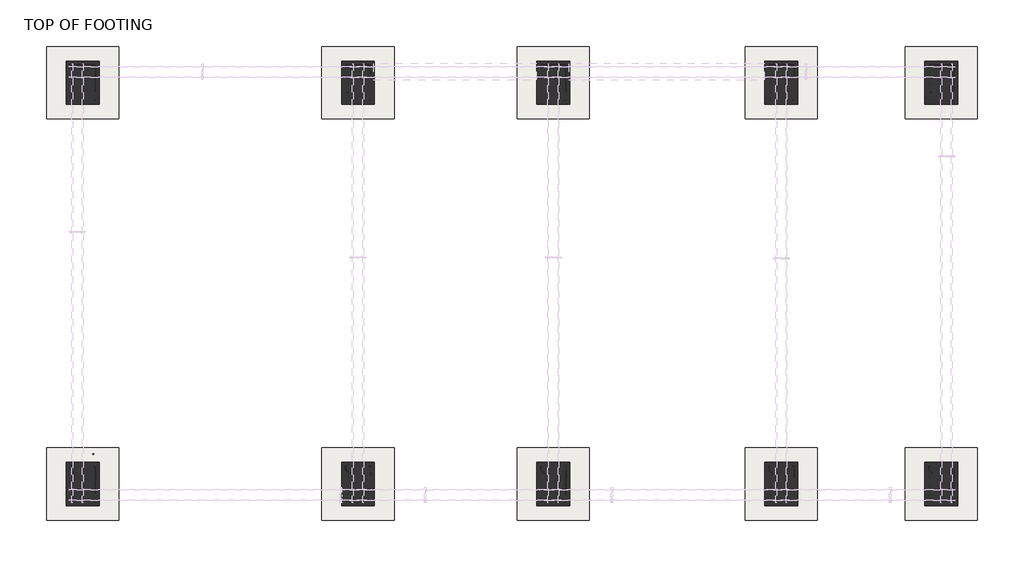
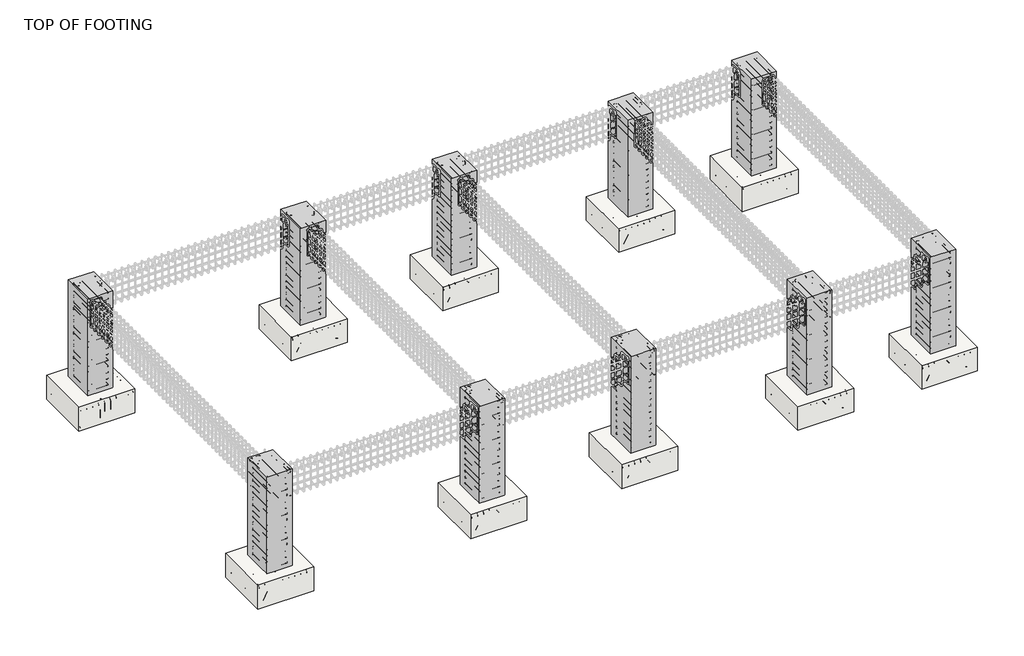
# One storey, part 1 of 9: 10 columns, 10 slabs.
"""IFC4 building model written with IfcOpenShell, lengths in millimetres."""

from ifc_helpers import new_model, si_unit, frame, origin, place, context, project, spatial, polyline, outline, extrude, transform, mapped, element, save
from components import m_footing_rectangular_1m_x_1m_x_450mm_4c97ae35

model = new_model("IFC4")

# Units and contexts
model_context = context("Model", 3, world=origin())
ifc_project = project(units=[si_unit("LENGTHUNIT", "METRE", prefix="MILLI")], contexts=[model_context])

# Site, building, storey
site = spatial("IfcSite", under=ifc_project)
building = spatial("IfcBuilding", under=site)
storey = spatial("IfcBuildingStorey", under=building, Name="TOP OF FOOTING", Elevation=-1828.8)

# Columns
placement = place(None, origin())
element("IfcColumn", 1, ObjectType="M_Concrete-Rectangular-Column : 450 x 600mm", at=placement, inside=storey, context=model_context, shape_type="SweptSolid", body=[
    extrude(outline(polyline([(-11358.2674526, 4792.8375236), (-11358.2674526, 4192.8375236), (-11808.2674526, 4192.8375236), (-11808.2674526, 4792.8375236), (-11358.2674526, 4792.8375236)])), frame((0.0, 0.0, -1828.8), z_axis=(0.0, 0.0, 1.0), x_axis=(1.0, 0.0, 0.0)), (0.0, 0.0, 1.0), 1828.8),
])
element("IfcColumn", 2, ObjectType="M_Concrete-Rectangular-Column : 450 x 600mm", at=placement, inside=storey, context=model_context, shape_type="SweptSolid", body=[
    extrude(outline(polyline([(-7558.2674526, 4792.8375236), (-7558.2674526, 4192.8375236), (-8008.2674526, 4192.8375236), (-8008.2674526, 4792.8375236), (-7558.2674526, 4792.8375236)])), frame((0.0, 0.0, -1828.8), z_axis=(0.0, 0.0, 1.0), x_axis=(1.0, 0.0, 0.0)), (0.0, 0.0, 1.0), 1828.8),
])
element("IfcColumn", 3, ObjectType="M_Concrete-Rectangular-Column : 450 x 600mm", at=placement, inside=storey, context=model_context, shape_type="SweptSolid", body=[
    extrude(outline(polyline([(-4858.2674526, 4792.8375236), (-4858.2674526, 4192.8375236), (-5308.2674526, 4192.8375236), (-5308.2674526, 4792.8375236), (-4858.2674526, 4792.8375236)])), frame((0.0, 0.0, -1828.8), z_axis=(0.0, 0.0, 1.0), x_axis=(1.0, 0.0, 0.0)), (0.0, 0.0, 1.0), 1828.8),
])
element("IfcColumn", 4, ObjectType="M_Concrete-Rectangular-Column : 450 x 600mm", at=placement, inside=storey, context=model_context, shape_type="SweptSolid", body=[
    extrude(outline(polyline([(-1708.2674526, 4792.8375236), (-1708.2674526, 4192.8375236), (-2158.2674526, 4192.8375236), (-2158.2674526, 4792.8375236), (-1708.2674526, 4792.8375236)])), frame((0.0, 0.0, -1828.8), z_axis=(0.0, 0.0, 1.0), x_axis=(1.0, 0.0, 0.0)), (0.0, 0.0, 1.0), 1828.8),
])
element("IfcColumn", 5, ObjectType="M_Concrete-Rectangular-Column : 450 x 600mm", at=placement, inside=storey, context=model_context, shape_type="SweptSolid", body=[
    extrude(outline(polyline([(501.7325474, 4792.8375236), (501.7325474, 4192.8375236), (51.7325474, 4192.8375236), (51.7325474, 4792.8375236), (501.7325474, 4792.8375236)])), frame((0.0, 0.0, -1828.8), z_axis=(0.0, 0.0, 1.0), x_axis=(1.0, 0.0, 0.0)), (0.0, 0.0, 1.0), 1828.8),
])
element("IfcColumn", 6, ObjectType="M_Concrete-Rectangular-Column : 450 x 600mm", at=placement, inside=storey, context=model_context, shape_type="SweptSolid", body=[
    extrude(outline(polyline([(-11358.2674526, -752.3324927), (-11358.2674526, -1352.3324927), (-11808.2674526, -1352.3324927), (-11808.2674526, -752.3324927), (-11358.2674526, -752.3324927)])), frame((0.0, 0.0, -1828.8), z_axis=(0.0, 0.0, 1.0), x_axis=(1.0, 0.0, 0.0)), (0.0, 0.0, 1.0), 1828.8),
])
element("IfcColumn", 7, ObjectType="M_Concrete-Rectangular-Column : 450 x 600mm", at=placement, inside=storey, context=model_context, shape_type="SweptSolid", body=[
    extrude(outline(polyline([(-7558.2674526, -752.3324927), (-7558.2674526, -1352.3324927), (-8008.2674526, -1352.3324927), (-8008.2674526, -752.3324927), (-7558.2674526, -752.3324927)])), frame((0.0, 0.0, -1828.8), z_axis=(0.0, 0.0, 1.0), x_axis=(1.0, 0.0, 0.0)), (0.0, 0.0, 1.0), 1828.8),
])
element("IfcColumn", 8, ObjectType="M_Concrete-Rectangular-Column : 450 x 600mm", at=placement, inside=storey, context=model_context, shape_type="SweptSolid", body=[
    extrude(outline(polyline([(-4858.2674526, -752.3324927), (-4858.2674526, -1352.3324927), (-5308.2674526, -1352.3324927), (-5308.2674526, -752.3324927), (-4858.2674526, -752.3324927)])), frame((0.0, 0.0, -1828.8), z_axis=(0.0, 0.0, 1.0), x_axis=(1.0, 0.0, 0.0)), (0.0, 0.0, 1.0), 1828.8),
])
element("IfcColumn", 9, ObjectType="M_Concrete-Rectangular-Column : 450 x 600mm", at=placement, inside=storey, context=model_context, shape_type="SweptSolid", body=[
    extrude(outline(polyline([(-1708.2674526, -752.3324927), (-1708.2674526, -1352.3324927), (-2158.2674526, -1352.3324927), (-2158.2674526, -752.3324927), (-1708.2674526, -752.3324927)])), frame((0.0, 0.0, -1828.8), z_axis=(0.0, 0.0, 1.0), x_axis=(1.0, 0.0, 0.0)), (0.0, 0.0, 1.0), 1828.8),
])
element("IfcColumn", 10, ObjectType="M_Concrete-Rectangular-Column : 450 x 600mm", at=placement, inside=storey, context=model_context, shape_type="SweptSolid", body=[
    extrude(outline(polyline([(501.7325474, -752.3324927), (501.7325474, -1352.3324927), (51.7325474, -1352.3324927), (51.7325474, -752.3324927), (501.7325474, -752.3324927)])), frame((0.0, 0.0, -1828.8), z_axis=(0.0, 0.0, 1.0), x_axis=(1.0, 0.0, 0.0)), (0.0, 0.0, 1.0), 1828.8),
])

# Slabs
m_footing_rectangular_1m_x_1m_x_450mm_shape = m_footing_rectangular_1m_x_1m_x_450mm_4c97ae35(model_context)
element("IfcSlab", 11, ObjectType="M_Footing-Rectangular : 1M X 1M X 450MM", at=placement, inside=storey, context=model_context, shape_type="MappedRepresentation", body=[
    mapped(m_footing_rectangular_1m_x_1m_x_450mm_shape, transform((-11583.2674526, 4492.8375236, -1828.8), x_axis=(1.0, 0.0, 0.0), y_axis=(0.0, 1.0, 0.0), z_axis=(0.0, 0.0, 1.0))),
])
element("IfcSlab", 12, ObjectType="M_Footing-Rectangular : 1M X 1M X 450MM", at=placement, inside=storey, context=model_context, shape_type="MappedRepresentation", body=[
    mapped(m_footing_rectangular_1m_x_1m_x_450mm_shape, transform((-7783.2674526, 4492.8375236, -1828.8), x_axis=(1.0, 0.0, 0.0), y_axis=(0.0, 1.0, 0.0), z_axis=(0.0, 0.0, 1.0))),
])
element("IfcSlab", 13, ObjectType="M_Footing-Rectangular : 1M X 1M X 450MM", at=placement, inside=storey, context=model_context, shape_type="MappedRepresentation", body=[
    mapped(m_footing_rectangular_1m_x_1m_x_450mm_shape, transform((-1933.2674526, 4492.8375236, -1828.8), x_axis=(1.0, 0.0, 0.0), y_axis=(0.0, 1.0, 0.0), z_axis=(0.0, 0.0, 1.0))),
])
element("IfcSlab", 14, ObjectType="M_Footing-Rectangular : 1M X 1M X 450MM", at=placement, inside=storey, context=model_context, shape_type="MappedRepresentation", body=[
    mapped(m_footing_rectangular_1m_x_1m_x_450mm_shape, transform((276.7325474, 4492.8375236, -1828.8), x_axis=(1.0, 0.0, 0.0), y_axis=(0.0, 1.0, 0.0), z_axis=(0.0, 0.0, 1.0))),
])
element("IfcSlab", 15, ObjectType="M_Footing-Rectangular : 1M X 1M X 450MM", at=placement, inside=storey, context=model_context, shape_type="MappedRepresentation", body=[
    mapped(m_footing_rectangular_1m_x_1m_x_450mm_shape, transform((-5083.2674526, 4492.8375236, -1828.8), x_axis=(1.0, 0.0, 0.0), y_axis=(0.0, 1.0, 0.0), z_axis=(0.0, 0.0, 1.0))),
])
element("IfcSlab", 16, ObjectType="M_Footing-Rectangular : 1M X 1M X 450MM", at=placement, inside=storey, context=model_context, shape_type="MappedRepresentation", body=[
    mapped(m_footing_rectangular_1m_x_1m_x_450mm_shape, transform((-11583.2674526, -1052.3324927, -1828.8), x_axis=(1.0, 0.0, 0.0), y_axis=(0.0, 1.0, 0.0), z_axis=(0.0, 0.0, 1.0))),
])
element("IfcSlab", 17, ObjectType="M_Footing-Rectangular : 1M X 1M X 450MM", at=placement, inside=storey, context=model_context, shape_type="MappedRepresentation", body=[
    mapped(m_footing_rectangular_1m_x_1m_x_450mm_shape, transform((-7783.2674526, -1052.3324927, -1828.8), x_axis=(1.0, 0.0, 0.0), y_axis=(0.0, 1.0, 0.0), z_axis=(0.0, 0.0, 1.0))),
])
element("IfcSlab", 18, ObjectType="M_Footing-Rectangular : 1M X 1M X 450MM", at=placement, inside=storey, context=model_context, shape_type="MappedRepresentation", body=[
    mapped(m_footing_rectangular_1m_x_1m_x_450mm_shape, transform((-5083.2674526, -1052.3324927, -1828.8), x_axis=(1.0, 0.0, 0.0), y_axis=(0.0, 1.0, 0.0), z_axis=(0.0, 0.0, 1.0))),
])
element("IfcSlab", 19, ObjectType="M_Footing-Rectangular : 1M X 1M X 450MM", at=placement, inside=storey, context=model_context, shape_type="MappedRepresentation", body=[
    mapped(m_footing_rectangular_1m_x_1m_x_450mm_shape, transform((-1933.2674526, -1052.3324927, -1828.8), x_axis=(1.0, 0.0, 0.0), y_axis=(0.0, 1.0, 0.0), z_axis=(0.0, 0.0, 1.0))),
])
element("IfcSlab", 20, ObjectType="M_Footing-Rectangular : 1M X 1M X 450MM", at=placement, inside=storey, context=model_context, shape_type="MappedRepresentation", body=[
    mapped(m_footing_rectangular_1m_x_1m_x_450mm_shape, transform((276.7325474, -1052.3324927, -1828.8), x_axis=(1.0, 0.0, 0.0), y_axis=(0.0, 1.0, 0.0), z_axis=(0.0, 0.0, 1.0))),
])

save(model, "model.ifc")

# Revit data of these elements
# Grids (mm)
#   "A": line (-11583.267, 9725.89) -> (-11583.267, -9561.893)
#   "B": line (-7783.267, 9725.89) -> (-7783.267, -9561.893)
#   "C": line (-5083.267, 9725.89) -> (-5083.267, -9561.893)
#   "D": line (-1933.267, 9725.89) -> (-1933.267, -9561.893)
#   "E": line (276.733, 9725.89) -> (276.733, -9561.893)
#   "1": line (2630.78, -1052.332) -> (-13801.455, -1052.332)
#   "2": line (2630.78, 4492.838) -> (-13801.455, 4492.838)
# Type "M_Concrete-Rectangular-Column : 450 x 600mm"
#   b = 450 mm
#   h = 600 mm
#   Structural Material [instance default] = Concrete, Cast-in-Place gray
# Type "M_Footing-Rectangular : 1M X 1M X 450MM"
#   Width = 1000 mm
#   Length = 1000 mm
#   Foundation Thickness = 450 mm
#   Structural Material [instance default] = Concrete, Cast-in-Place gray
#   Assembly Code = ""
# Elements 1, 2, 3, 4, 5, 6, 7, 8, 9, 10 (IfcColumn, "M_Concrete-Rectangular-Column : 450 x 600mm")
#   Structural Material = Concrete, Cast-in-Place gray
#   Phase Created = New Construction
#   Materials on its faces: "Concrete, Cast-in-Place gray"
# Elements 11, 12, 13, 14, 15, 16, 17, 18, 19, 20 (IfcSlab, "M_Footing-Rectangular : 1M X 1M X 450MM")
#   Structural Material = Concrete, Cast-in-Place gray
#   Phase Created = New Construction
#   Materials on its faces: "Concrete, Cast-in-Place gray"
# Materials
#   "Concrete, Cast-in-Place gray": class "Concrete", colour RGB 192 192 192, transparency 0, Description = "Cast-in-place concrete", Cost = 0
